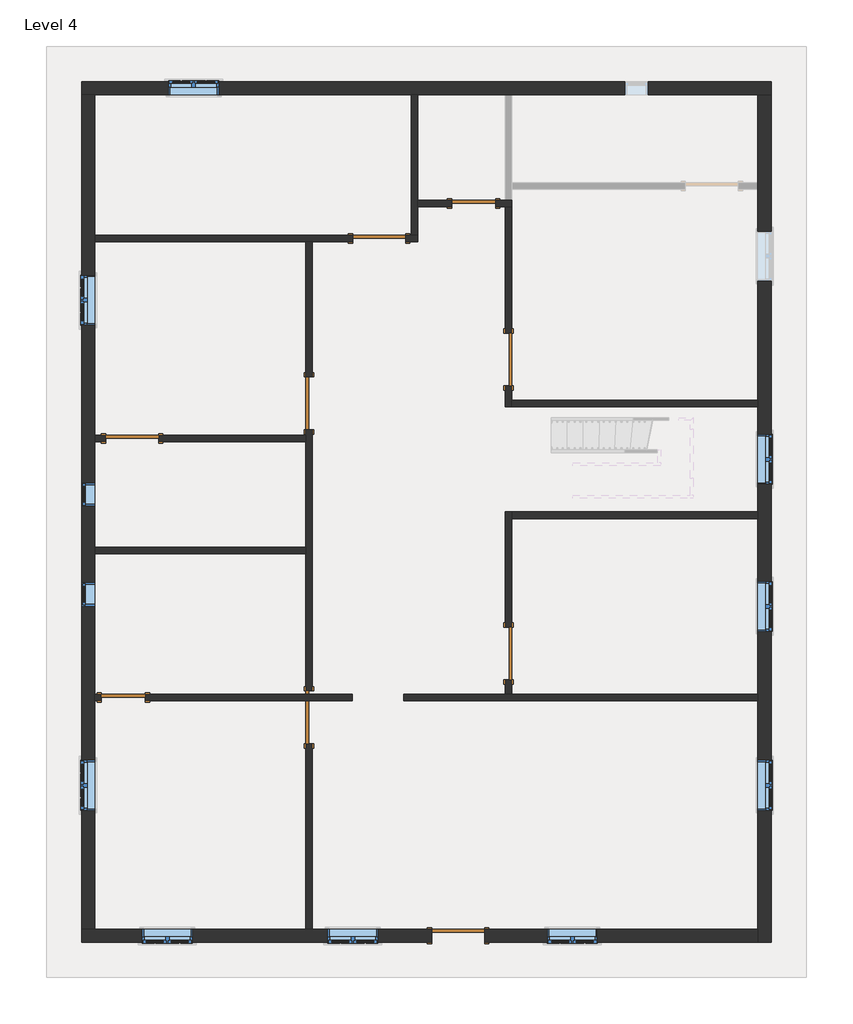
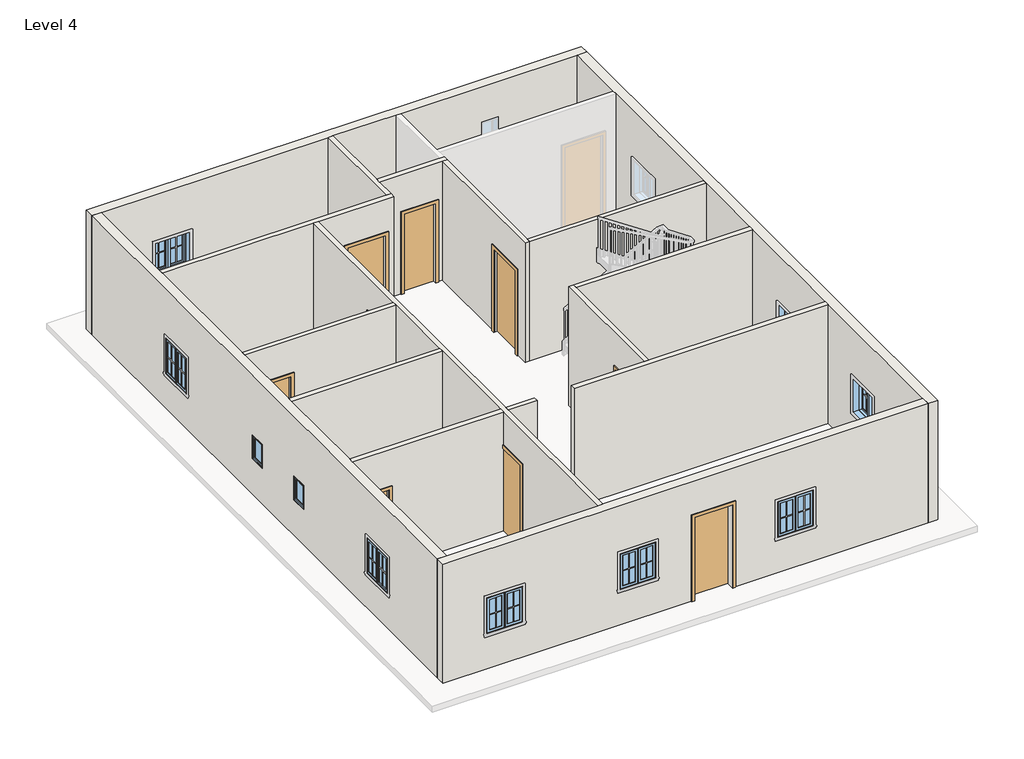
# One storey, part 1 of 3: 16 walls, 11 windows, 9 doors.
"""IFC4 building model written with IfcOpenShell, lengths in millimetres."""

from ifc_helpers import new_model, si_unit, frame, origin, place, context, project, spatial, polyline, outline, extrude, faceted_brep, transform, mapped, element, save
from components import door_d8f5dbb5, door_f2b275c1, door_e5f9f3c4, door_305aa2a5, door_a90ba1ad, window_aa618e30, window_339605e1

model = new_model("IFC4")

# Units and contexts
model_context = context("Model", 3, world=origin())
ifc_project = project(units=[si_unit("LENGTHUNIT", "METRE", prefix="MILLI")], contexts=[model_context])

# Site, building, storey
site = spatial("IfcSite", under=ifc_project)
building = spatial("IfcBuilding", under=site)
storey = spatial("IfcBuildingStorey", under=building, Name="Level 4", Elevation=6400.8)

# Doors
placement = place(None, origin())
door_shape = door_d8f5dbb5(model_context)
element("IfcDoor", 1, ObjectType="Single-Flush : 30\" x 80\"", at=placement, inside=storey, context=model_context, shape_type="MappedRepresentation", body=[
    mapped(door_shape, transform((-509.1743007, 6967.427558, 6400.8), x_axis=(1.0, 0.0, 0.0), y_axis=(0.0, 1.0, 0.0), z_axis=(0.0, 0.0, 1.0))),
])
door_2_shape = door_f2b275c1(model_context)
element("IfcDoor", 2, ObjectType="Single-Flush : 30\" x 80\"", at=placement, inside=storey, context=model_context, shape_type="MappedRepresentation", body=[
    mapped(door_2_shape, transform((-6586.1243007, -1605.072442, 6400.8), x_axis=(-1.0, 0.0, 0.0), y_axis=(0.0, -1.0, 0.0), z_axis=(0.0, 0.0, 1.0))),
])
door_3_shape = door_e5f9f3c4(model_context)
element("IfcDoor", 3, ObjectType="Single-Flush : 36\" x 84\"", at=placement, inside=storey, context=model_context, shape_type="MappedRepresentation", body=[
    mapped(door_3_shape, transform((-2147.4743007, 6357.827558, 6400.8), x_axis=(1.0, 0.0, 0.0), y_axis=(0.0, 1.0, 0.0), z_axis=(0.0, 0.0, 1.0))),
])
element("IfcDoor", 4, ObjectType="Single-Flush : 36\" x 84\"", at=placement, inside=storey, context=model_context, shape_type="MappedRepresentation", body=[
    mapped(door_3_shape, transform((100.4256993, 4262.327558, 6400.8), x_axis=(0.0, -1.0, 0.0), y_axis=(1.0, 0.0, 0.0), z_axis=(0.0, 0.0, 1.0))),
])
element("IfcDoor", 5, ObjectType="Single-Flush : 36\" x 84\"", at=placement, inside=storey, context=model_context, shape_type="MappedRepresentation", body=[
    mapped(door_3_shape, transform((100.4256993, -843.072442, 6400.8), x_axis=(0.0, -1.0, 0.0), y_axis=(1.0, 0.0, 0.0), z_axis=(0.0, 0.0, 1.0))),
])
element("IfcDoor", 6, ObjectType="Single-Flush : 36\" x 84\"", at=placement, inside=storey, context=model_context, shape_type="MappedRepresentation", body=[
    mapped(door_3_shape, transform((-3366.6743007, -1947.972442, 6400.8), x_axis=(0.0, 1.0, 0.0), y_axis=(-1.0, 0.0, 0.0), z_axis=(0.0, 0.0, 1.0))),
])
door_4_shape = door_305aa2a5(model_context)
element("IfcDoor", 7, ObjectType="Single-Flush : 36\" x 84\"", at=placement, inside=storey, context=model_context, shape_type="MappedRepresentation", body=[
    mapped(door_4_shape, transform((-6433.7243007, 2890.727558, 6400.8), x_axis=(-1.0, 0.0, 0.0), y_axis=(0.0, -1.0, 0.0), z_axis=(0.0, 0.0, 1.0))),
])
element("IfcDoor", 8, ObjectType="Single-Flush : 36\" x 84\"", at=placement, inside=storey, context=model_context, shape_type="MappedRepresentation", body=[
    mapped(door_4_shape, transform((-3366.6743007, 3500.327558, 6400.8), x_axis=(0.0, -1.0, 0.0), y_axis=(1.0, 0.0, 0.0), z_axis=(0.0, 0.0, 1.0))),
])
door_5_shape = door_a90ba1ad(model_context)
element("IfcDoor", 9, ObjectType="Single-Flush : 36\" x 84\"", at=placement, inside=storey, context=model_context, shape_type="MappedRepresentation", body=[
    mapped(door_5_shape, transform((-775.8743007, -5738.922442, 6400.8), x_axis=(-1.0, 0.0, 0.0), y_axis=(0.0, -1.0, 0.0), z_axis=(0.0, 0.0, 1.0))),
])

# Walls
element("IfcWall", 10, ObjectType="WALL4.5\"", at=placement, inside=storey, context=model_context, shape_type="Brep", body=[
    faceted_brep([(-1690.2743007, 6300.677558, 8534.4), (-1690.2743007, 6300.677558, 6400.8), (-1480.7243007, 6300.677558, 6400.8), (-1480.7243007, 6300.677558, 9448.8), (-3309.5243007, 6300.677558, 9448.8), (-3423.8243007, 6300.677558, 9448.8), (-7081.4243007, 6300.677558, 9448.8), (-7081.4243007, 6300.677558, 6400.8), (-3423.8243007, 6300.677558, 6400.8), (-3309.5243007, 6300.677558, 6400.8), (-2604.6743007, 6300.677558, 6400.8), (-2604.6743007, 6300.677558, 8534.4), (-1480.7243007, 6414.977558, 6400.8), (-1595.0243007, 6414.977558, 6400.8), (-1690.2743007, 6414.977558, 6400.8), (-1690.2743007, 6414.977558, 8534.4), (-2604.6743007, 6414.977558, 8534.4), (-2604.6743007, 6414.977558, 6400.8), (-7081.4243007, 6414.977558, 6400.8), (-7081.4243007, 6414.977558, 9448.8), (-1595.0243007, 6414.977558, 9448.8), (-1480.7243007, 6414.977558, 9448.8)], [[[0, 1, 2, 3, 4, 5, 6, 7, 8, 9, 10, 11]], [[12, 13, 14, 15, 16, 17, 18, 19, 20, 21]], [[2, 1, 14, 13, 12]], [[10, 9, 8, 7, 18, 17]], [[7, 6, 19, 18]], [[3, 2, 12, 21]], [[15, 14, 1, 0]], [[16, 15, 0, 11]], [[17, 16, 11, 10]], [[6, 5, 4, 3, 21, 20, 19]]]),
])
element("IfcWall", 11, ObjectType="WALL4.5\"", at=placement, inside=storey, context=model_context, shape_type="Brep", body=[
    faceted_brep([(-1480.7243007, 6414.977558, 6400.8), (-1480.7243007, 6910.277558, 6400.8), (-1480.7243007, 7024.577558, 6400.8), (-1480.7243007, 8853.377558, 6400.8), (-1480.7243007, 8853.377558, 9448.8), (-1480.7243007, 7024.577558, 9448.8), (-1480.7243007, 6910.277558, 9448.8), (-1480.7243007, 6414.977558, 9448.8), (-1595.0243007, 6414.977558, 6400.8), (-1595.0243007, 6414.977558, 9448.8), (-1595.0243007, 8853.377558, 9448.8), (-1595.0243007, 8853.377558, 6400.8)], [[[0, 1, 2, 3, 4, 5, 6, 7]], [[8, 9, 10, 11]], [[3, 2, 1, 0, 8, 11]], [[0, 7, 9, 8]], [[4, 3, 11, 10]], [[7, 6, 5, 4, 10, 9]]]),
])
element("IfcWall", 12, ObjectType="WALL4.5\"", at=placement, inside=storey, context=model_context, shape_type="Brep", body=[
    faceted_brep([(-128.1743007, 6910.277558, 8432.8), (-128.1743007, 6910.277558, 6400.8), (43.2756993, 6910.277558, 6400.8), (157.5756993, 6910.277558, 6400.8), (157.5756993, 6910.277558, 9448.8), (43.2756993, 6910.277558, 9448.8), (-1480.7243007, 6910.277558, 9448.8), (-1480.7243007, 6910.277558, 6400.8), (-890.1743007, 6910.277558, 6400.8), (-890.1743007, 6910.277558, 8432.8), (157.5756993, 7024.577558, 6400.8), (43.2756993, 7024.577558, 6400.8), (-128.1743007, 7024.577558, 6400.8), (-128.1743007, 7024.577558, 8432.8), (-890.1743007, 7024.577558, 8432.8), (-890.1743007, 7024.577558, 6400.8), (-1480.7243007, 7024.577558, 6400.8), (-1480.7243007, 7024.577558, 9448.8), (43.2756993, 7024.577558, 9448.8), (157.5756993, 7024.577558, 9448.8)], [[[0, 1, 2, 3, 4, 5, 6, 7, 8, 9]], [[10, 11, 12, 13, 14, 15, 16, 17, 18, 19]], [[8, 7, 16, 15]], [[3, 2, 1, 12, 11, 10]], [[7, 6, 17, 16]], [[4, 3, 10, 19]], [[13, 12, 1, 0]], [[14, 13, 0, 9]], [[15, 14, 9, 8]], [[6, 5, 4, 19, 18, 17]]]),
])
element("IfcWall", 13, ObjectType="WALL4.5\"", at=placement, inside=storey, context=model_context, shape_type="Brep", body=[
    faceted_brep([(-3423.8243007, 3043.127558, 6400.8), (-3423.8243007, 2947.877558, 6400.8), (-3423.8243007, 2833.577558, 6400.8), (-3423.8243007, 1004.777558, 6400.8), (-3423.8243007, 890.477558, 6400.8), (-3423.8243007, -1490.772442, 6400.8), (-3423.8243007, -1490.772442, 8534.4), (-3423.8243007, -1547.922442, 8534.4), (-3423.8243007, -1662.222442, 8534.4), (-3423.8243007, -2405.172442, 8534.4), (-3423.8243007, -2405.172442, 6400.8), (-3423.8243007, -5624.622442, 6400.8), (-3423.8243007, -5624.622442, 9448.8), (-3423.8243007, -1662.222442, 9448.8), (-3423.8243007, -1547.922442, 9448.8), (-3423.8243007, 890.477558, 9448.8), (-3423.8243007, 1004.777558, 9448.8), (-3423.8243007, 2833.577558, 9448.8), (-3423.8243007, 2947.877558, 9448.8), (-3423.8243007, 6300.677558, 9448.8), (-3423.8243007, 6300.677558, 6400.8), (-3423.8243007, 3957.527558, 6400.8), (-3423.8243007, 3957.527558, 8534.4), (-3423.8243007, 3043.127558, 8534.4), (-3309.5243007, -1490.772442, 8534.4), (-3309.5243007, -1490.772442, 6400.8), (-3309.5243007, 3043.127558, 6400.8), (-3309.5243007, 3043.127558, 8534.4), (-3309.5243007, 3957.527558, 8534.4), (-3309.5243007, 3957.527558, 6400.8), (-3309.5243007, 6300.677558, 6400.8), (-3309.5243007, 6300.677558, 9448.8), (-3309.5243007, -1547.922442, 9448.8), (-3309.5243007, -1662.222442, 9448.8), (-3309.5243007, -5624.622442, 9448.8), (-3309.5243007, -5624.622442, 6400.8), (-3309.5243007, -2405.172442, 6400.8), (-3309.5243007, -2405.172442, 8534.4), (-3309.5243007, -1662.222442, 8534.4), (-3309.5243007, -1547.922442, 8534.4)], [[[0, 1, 2, 3, 4, 5, 6, 7, 8, 9, 10, 11, 12, 13, 14, 15, 16, 17, 18, 19, 20, 21, 22, 23]], [[24, 25, 26, 27, 28, 29, 30, 31, 32, 33, 34, 35, 36, 37, 38, 39]], [[21, 20, 30, 29]], [[36, 35, 11, 10]], [[26, 25, 5, 4, 3, 2, 1, 0]], [[12, 11, 35, 34]], [[20, 19, 31, 30]], [[27, 26, 0, 23]], [[28, 27, 23, 22]], [[29, 28, 22, 21]], [[6, 5, 25, 24]], [[9, 8, 7, 6, 24, 39, 38, 37]], [[10, 9, 37, 36]], [[19, 18, 17, 16, 15, 14, 13, 12, 34, 33, 32, 31]]]),
])
element("IfcWall", 14, ObjectType="WALL4.5\"", at=placement, inside=storey, context=model_context, shape_type="Brep", body=[
    faceted_brep([(157.5756993, -1547.922442, 6400.8), (157.5756993, -1300.272442, 6400.8), (157.5756993, -1300.272442, 8534.4), (157.5756993, -385.872442, 8534.4), (157.5756993, -385.872442, 6400.8), (157.5756993, 1500.077558, 6400.8), (157.5756993, 1614.377558, 6400.8), (157.5756993, 1614.377558, 9448.8), (157.5756993, 1500.077558, 9448.8), (157.5756993, -1547.922442, 9448.8), (43.2756993, -1300.272442, 8534.4), (43.2756993, -1300.272442, 6400.8), (43.2756993, -1547.922442, 6400.8), (43.2756993, -1547.922442, 9448.8), (43.2756993, 1614.377558, 9448.8), (43.2756993, 1614.377558, 6400.8), (43.2756993, -385.872442, 6400.8), (43.2756993, -385.872442, 8534.4)], [[[0, 1, 2, 3, 4, 5, 6, 7, 8, 9]], [[10, 11, 12, 13, 14, 15, 16, 17]], [[16, 15, 6, 5, 4]], [[12, 11, 1, 0]], [[7, 6, 15, 14]], [[0, 9, 13, 12]], [[2, 1, 11, 10]], [[3, 2, 10, 17]], [[4, 3, 17, 16]], [[9, 8, 7, 14, 13]]]),
])
element("IfcWall", 15, ObjectType="WALL4.5\"", at=placement, inside=storey, context=model_context, shape_type="SweptSolid", body=[
    extrude(outline(polyline([(4424.7756993, 1500.077558), (157.5756993, 1500.077558), (157.5756993, 1614.377558), (4424.7756993, 1614.377558), (4424.7756993, 1500.077558)])), frame((0.0, 0.0, 6400.8), z_axis=(0.0, 0.0, 1.0), x_axis=(1.0, 0.0, 0.0)), (0.0, 0.0, 1.0), 3048.0),
])
element("IfcWall", 16, ObjectType="WALL4.5\"", at=placement, inside=storey, context=model_context, shape_type="SweptSolid", body=[
    extrude(outline(polyline([(-3423.8243007, 890.477558), (-7081.4243007, 890.477558), (-7081.4243007, 1004.777558), (-3423.8243007, 1004.777558), (-3423.8243007, 890.477558)])), frame((0.0, 0.0, 6400.8), z_axis=(0.0, 0.0, 1.0), x_axis=(1.0, 0.0, 0.0)), (0.0, 0.0, 1.0), 3048.0),
])
element("IfcWall", 17, ObjectType="WALL4.5\"", at=placement, inside=storey, context=model_context, shape_type="SweptSolid", body=[
    extrude(outline(polyline([(6400.8, -7081.4243007), (6400.8, -6890.9243007), (8534.4, -6890.9243007), (8534.4, -5976.5243007), (6400.8, -5976.5243007), (6400.8, -3423.8243007), (9448.8, -3423.8243007), (9448.8, -7081.4243007), (6400.8, -7081.4243007)])), frame((0.0, 2833.577558, 0.0), z_axis=(0.0, 1.0, 0.0), x_axis=(0.0, 0.0, 1.0)), (0.0, 0.0, 1.0), 114.3),
])
element("IfcWall", 18, ObjectType="WALL4.5\"", at=placement, inside=storey, context=model_context, shape_type="Brep", body=[
    faceted_brep([(43.2756993, 3805.127558, 8534.4), (43.2756993, 3805.127558, 6400.8), (43.2756993, 3443.177558, 6400.8), (43.2756993, 3443.177558, 9448.8), (43.2756993, 6910.277558, 9448.8), (43.2756993, 6910.277558, 6400.8), (43.2756993, 4719.527558, 6400.8), (43.2756993, 4719.527558, 8534.4), (157.5756993, 3443.177558, 6400.8), (157.5756993, 3557.477558, 6400.8), (157.5756993, 3805.127558, 6400.8), (157.5756993, 3805.127558, 8534.4), (157.5756993, 4719.527558, 8534.4), (157.5756993, 4719.527558, 6400.8), (157.5756993, 6910.277558, 6400.8), (157.5756993, 6910.277558, 9448.8), (157.5756993, 3557.477558, 9448.8), (157.5756993, 3443.177558, 9448.8)], [[[0, 1, 2, 3, 4, 5, 6, 7]], [[8, 9, 10, 11, 12, 13, 14, 15, 16, 17]], [[6, 5, 14, 13]], [[2, 1, 10, 9, 8]], [[5, 4, 15, 14]], [[3, 2, 8, 17]], [[11, 10, 1, 0]], [[12, 11, 0, 7]], [[13, 12, 7, 6]], [[4, 3, 17, 16, 15]]]),
])
element("IfcWall", 19, ObjectType="WALL4.5\"", at=placement, inside=storey, context=model_context, shape_type="SweptSolid", body=[
    extrude(outline(polyline([(4424.7756993, 3443.177558), (157.5756993, 3443.177558), (157.5756993, 3557.477558), (4424.7756993, 3557.477558), (4424.7756993, 3443.177558)])), frame((0.0, 0.0, 6400.8), z_axis=(0.0, 0.0, 1.0), x_axis=(1.0, 0.0, 0.0)), (0.0, 0.0, 1.0), 3048.0),
])
element("IfcWall", 20, ObjectType="WALL4.5\"", at=placement, inside=storey, context=model_context, shape_type="SweptSolid", body=[
    extrude(outline(polyline([(6400.8, -2614.8628774), (9448.8, -2614.8628774), (9448.8, -3309.5243007), (8534.4, -3309.5243007), (8534.4, -3423.8243007), (9448.8, -3423.8243007), (9448.8, -7081.4243007), (6400.8, -7081.4243007), (6400.8, -6967.1243007), (8432.8, -6967.1243007), (8432.8, -6205.1243007), (6400.8, -6205.1243007), (6400.8, -2614.8628774)])), frame((0.0, -1662.222442, 0.0), z_axis=(0.0, 1.0, 0.0), x_axis=(0.0, 0.0, 1.0)), (0.0, 0.0, 1.0), 114.3),
])
element("IfcWall", 21, ObjectType="WALL4.5\"", at=placement, inside=storey, context=model_context, shape_type="Brep", body=[
    faceted_brep([(-1720.6441625, -1662.222442, 6400.8), (4424.7756993, -1662.222442, 6400.8), (4424.7756993, -1662.222442, 9448.8), (-1720.6441625, -1662.222442, 9448.8), (-1720.6441625, -1547.922442, 6400.8), (-1720.6441625, -1547.922442, 9448.8), (43.2756993, -1547.922442, 9448.8), (157.5756993, -1547.922442, 9448.8), (4424.7756993, -1547.922442, 9448.8), (4424.7756993, -1547.922442, 6400.8), (157.5756993, -1547.922442, 6400.8), (43.2756993, -1547.922442, 6400.8)], [[[0, 1, 2, 3]], [[4, 5, 6, 7, 8, 9, 10, 11]], [[1, 0, 4, 11, 10, 9]], [[0, 3, 5, 4]], [[2, 1, 9, 8]], [[3, 2, 8, 7, 6, 5]]]),
])
element("IfcWall", 22, ObjectType="WALL9\"", at=placement, inside=storey, context=model_context, shape_type="Brep", body=[
    faceted_brep([(-7310.0243007, 8853.377558, 6400.8), (-7081.4243007, 8853.377558, 6400.8), (-1595.0243007, 8853.377558, 6400.8), (-1480.7243007, 8853.377558, 6400.8), (43.2756993, 8853.377558, 6400.8), (157.5756993, 8853.377558, 6400.8), (4424.7756993, 8853.377558, 6400.8), (4653.3756993, 8853.377558, 6400.8), (4653.3756993, 8853.377558, 9448.8), (4424.7756993, 8853.377558, 9448.8), (157.5756993, 8853.377558, 9448.8), (43.2756993, 8853.377558, 9448.8), (-1480.7243007, 8853.377558, 9448.8), (-1595.0243007, 8853.377558, 9448.8), (-7081.4243007, 8853.377558, 9448.8), (-7310.0243007, 8853.377558, 9448.8), (-4935.1243007, 8853.377558, 8229.6), (-4935.1243007, 8853.377558, 7315.2), (-5798.7243007, 8853.377558, 7315.2), (-5798.7243007, 8853.377558, 8229.6), (2522.9506993, 8853.377558, 8534.4), (2522.9506993, 8853.377558, 6705.6), (2116.5506993, 8853.377558, 6705.6), (2116.5506993, 8853.377558, 8534.4), (-7310.0243007, 9081.977558, 6400.8), (-7310.0243007, 9081.977558, 9448.8), (4653.3756993, 9081.977558, 9448.8), (4653.3756993, 9081.977558, 6400.8), (-4935.1243007, 9081.977558, 8229.6), (-5798.7243007, 9081.977558, 8229.6), (-5798.7243007, 9081.977558, 7315.2), (-4935.1243007, 9081.977558, 7315.2), (2522.9506993, 9081.977558, 8534.4), (2116.5506993, 9081.977558, 8534.4), (2116.5506993, 9081.977558, 6705.6), (2522.9506993, 9081.977558, 6705.6)], [[[0, 1, 2, 3, 4, 5, 6, 7, 8, 9, 10, 11, 12, 13, 14, 15], [16, 17, 18, 19], [20, 21, 22, 23]], [[24, 25, 26, 27], [28, 29, 30, 31], [32, 33, 34, 35]], [[7, 6, 5, 4, 3, 2, 1, 0, 24, 27]], [[8, 7, 27, 26]], [[0, 15, 25, 24]], [[17, 16, 28, 31]], [[18, 17, 31, 30]], [[19, 18, 30, 29]], [[16, 19, 29, 28]], [[21, 20, 32, 35]], [[22, 21, 35, 34]], [[23, 22, 34, 33]], [[20, 23, 33, 32]], [[15, 14, 13, 12, 11, 10, 9, 8, 26, 25]]]),
])
element("IfcWall", 23, ObjectType="WALL9\"", at=placement, inside=storey, context=model_context, shape_type="Brep", body=[
    faceted_brep([(4424.7756993, 8853.377558, 6400.8), (4424.7756993, 7329.377558, 6400.8), (4424.7756993, 7215.077558, 6400.8), (4424.7756993, 3557.477558, 6400.8), (4424.7756993, 3443.177558, 6400.8), (4424.7756993, 1614.377558, 6400.8), (4424.7756993, 1500.077558, 6400.8), (4424.7756993, -1547.922442, 6400.8), (4424.7756993, -1662.222442, 6400.8), (4424.7756993, -5624.622442, 6400.8), (4424.7756993, -5853.222442, 6400.8), (4424.7756993, -5853.222442, 9448.8), (4424.7756993, -5624.622442, 9448.8), (4424.7756993, -1662.222442, 9448.8), (4424.7756993, -1547.922442, 9448.8), (4424.7756993, 1500.077558, 9448.8), (4424.7756993, 1614.377558, 9448.8), (4424.7756993, 3443.177558, 9448.8), (4424.7756993, 3557.477558, 9448.8), (4424.7756993, 7215.077558, 9448.8), (4424.7756993, 7329.377558, 9448.8), (4424.7756993, 8853.377558, 9448.8), (4424.7756993, 5621.227558, 8229.6), (4424.7756993, 5621.227558, 7315.2), (4424.7756993, 6484.827558, 7315.2), (4424.7756993, 6484.827558, 8229.6), (4424.7756993, 2096.977558, 8229.6), (4424.7756993, 2096.977558, 7315.2), (4424.7756993, 2960.577558, 7315.2), (4424.7756993, 2960.577558, 8229.6), (4424.7756993, -455.722442, 8229.6), (4424.7756993, -455.722442, 7315.2), (4424.7756993, 407.877558, 7315.2), (4424.7756993, 407.877558, 8229.6), (4424.7756993, -3560.872442, 8229.6), (4424.7756993, -3560.872442, 7315.2), (4424.7756993, -2697.272442, 7315.2), (4424.7756993, -2697.272442, 8229.6), (4653.3756993, 8853.377558, 6400.8), (4653.3756993, 8853.377558, 9448.8), (4653.3756993, -5853.222442, 9448.8), (4653.3756993, -5853.222442, 6400.8), (4653.3756993, 5621.227558, 8229.6), (4653.3756993, 6484.827558, 8229.6), (4653.3756993, 6484.827558, 7315.2), (4653.3756993, 5621.227558, 7315.2), (4653.3756993, 2096.977558, 8229.6), (4653.3756993, 2960.577558, 8229.6), (4653.3756993, 2960.577558, 7315.2), (4653.3756993, 2096.977558, 7315.2), (4653.3756993, -455.722442, 8229.6), (4653.3756993, 407.877558, 8229.6), (4653.3756993, 407.877558, 7315.2), (4653.3756993, -455.722442, 7315.2), (4653.3756993, -3560.872442, 8229.6), (4653.3756993, -2697.272442, 8229.6), (4653.3756993, -2697.272442, 7315.2), (4653.3756993, -3560.872442, 7315.2)], [[[0, 1, 2, 3, 4, 5, 6, 7, 8, 9, 10, 11, 12, 13, 14, 15, 16, 17, 18, 19, 20, 21], [22, 23, 24, 25], [26, 27, 28, 29], [30, 31, 32, 33], [34, 35, 36, 37]], [[38, 39, 40, 41], [42, 43, 44, 45], [46, 47, 48, 49], [50, 51, 52, 53], [54, 55, 56, 57]], [[10, 9, 8, 7, 6, 5, 4, 3, 2, 1, 0, 38, 41]], [[0, 21, 39, 38]], [[11, 10, 41, 40]], [[23, 22, 42, 45]], [[24, 23, 45, 44]], [[25, 24, 44, 43]], [[22, 25, 43, 42]], [[27, 26, 46, 49]], [[28, 27, 49, 48]], [[29, 28, 48, 47]], [[26, 29, 47, 46]], [[31, 30, 50, 53]], [[32, 31, 53, 52]], [[33, 32, 52, 51]], [[30, 33, 51, 50]], [[35, 34, 54, 57]], [[36, 35, 57, 56]], [[37, 36, 56, 55]], [[34, 37, 55, 54]], [[21, 20, 19, 18, 17, 16, 15, 14, 13, 12, 11, 40, 39]]]),
])
element("IfcWall", 24, ObjectType="WALL9\"", at=placement, inside=storey, context=model_context, shape_type="Brep", body=[
    faceted_brep([(-1233.0743007, -5624.622442, 8534.4), (-1233.0743007, -5624.622442, 6400.8), (-3309.5243007, -5624.622442, 6400.8), (-3423.8243007, -5624.622442, 6400.8), (-7081.4243007, -5624.622442, 6400.8), (-7310.0243007, -5624.622442, 6400.8), (-7310.0243007, -5624.622442, 9448.8), (-7081.4243007, -5624.622442, 9448.8), (-3423.8243007, -5624.622442, 9448.8), (-3309.5243007, -5624.622442, 9448.8), (4424.7756993, -5624.622442, 9448.8), (4424.7756993, -5624.622442, 6400.8), (-318.6743007, -5624.622442, 6400.8), (-318.6743007, -5624.622442, 8534.4), (773.5256993, -5624.622442, 8229.6), (773.5256993, -5624.622442, 7315.2), (1637.1256993, -5624.622442, 7315.2), (1637.1256993, -5624.622442, 8229.6), (-3036.4743007, -5624.622442, 8229.6), (-3036.4743007, -5624.622442, 7315.2), (-2172.8743007, -5624.622442, 7315.2), (-2172.8743007, -5624.622442, 8229.6), (-6255.9243007, -5624.622442, 8229.6), (-6255.9243007, -5624.622442, 7315.2), (-5392.3243007, -5624.622442, 7315.2), (-5392.3243007, -5624.622442, 8229.6), (-7310.0243007, -5853.222442, 6400.8), (-1233.0743007, -5853.222442, 6400.8), (-1233.0743007, -5853.222442, 8534.4), (-318.6743007, -5853.222442, 8534.4), (-318.6743007, -5853.222442, 6400.8), (4424.7756993, -5853.222442, 6400.8), (4424.7756993, -5853.222442, 9448.8), (-7310.0243007, -5853.222442, 9448.8), (773.5256993, -5853.222442, 8229.6), (1637.1256993, -5853.222442, 8229.6), (1637.1256993, -5853.222442, 7315.2), (773.5256993, -5853.222442, 7315.2), (-3036.4743007, -5853.222442, 8229.6), (-2172.8743007, -5853.222442, 8229.6), (-2172.8743007, -5853.222442, 7315.2), (-3036.4743007, -5853.222442, 7315.2), (-6255.9243007, -5853.222442, 8229.6), (-5392.3243007, -5853.222442, 8229.6), (-5392.3243007, -5853.222442, 7315.2), (-6255.9243007, -5853.222442, 7315.2)], [[[0, 1, 2, 3, 4, 5, 6, 7, 8, 9, 10, 11, 12, 13], [14, 15, 16, 17], [18, 19, 20, 21], [22, 23, 24, 25]], [[26, 27, 28, 29, 30, 31, 32, 33], [34, 35, 36, 37], [38, 39, 40, 41], [42, 43, 44, 45]], [[12, 11, 31, 30]], [[5, 4, 3, 2, 1, 27, 26]], [[11, 10, 32, 31]], [[6, 5, 26, 33]], [[28, 27, 1, 0]], [[29, 28, 0, 13]], [[30, 29, 13, 12]], [[15, 14, 34, 37]], [[16, 15, 37, 36]], [[17, 16, 36, 35]], [[14, 17, 35, 34]], [[19, 18, 38, 41]], [[20, 19, 41, 40]], [[21, 20, 40, 39]], [[18, 21, 39, 38]], [[23, 22, 42, 45]], [[24, 23, 45, 44]], [[25, 24, 44, 43]], [[22, 25, 43, 42]], [[10, 9, 8, 7, 6, 33, 32]]]),
])
element("IfcWall", 25, ObjectType="WALL9\"", at=placement, inside=storey, context=model_context, shape_type="Brep", body=[
    faceted_brep([(-7081.4243007, -5624.622442, 6400.8), (-7081.4243007, -1662.222442, 6400.8), (-7081.4243007, -1547.922442, 6400.8), (-7081.4243007, 890.477558, 6400.8), (-7081.4243007, 1004.777558, 6400.8), (-7081.4243007, 2833.577558, 6400.8), (-7081.4243007, 2947.877558, 6400.8), (-7081.4243007, 6300.677558, 6400.8), (-7081.4243007, 6414.977558, 6400.8), (-7081.4243007, 8853.377558, 6400.8), (-7081.4243007, 8853.377558, 9448.8), (-7081.4243007, 6414.977558, 9448.8), (-7081.4243007, 6300.677558, 9448.8), (-7081.4243007, 2947.877558, 9448.8), (-7081.4243007, 2833.577558, 9448.8), (-7081.4243007, 1004.777558, 9448.8), (-7081.4243007, 890.477558, 9448.8), (-7081.4243007, -1547.922442, 9448.8), (-7081.4243007, -1662.222442, 9448.8), (-7081.4243007, -5624.622442, 9448.8), (-7081.4243007, 388.827558, 7924.8), (-7081.4243007, 388.827558, 7315.2), (-7081.4243007, -17.572442, 7315.2), (-7081.4243007, -17.572442, 7924.8), (-7081.4243007, 2122.377558, 7924.8), (-7081.4243007, 2122.377558, 7315.2), (-7081.4243007, 1715.977558, 7315.2), (-7081.4243007, 1715.977558, 7924.8), (-7081.4243007, 5722.827558, 8229.6), (-7081.4243007, 5722.827558, 7315.2), (-7081.4243007, 4859.227558, 7315.2), (-7081.4243007, 4859.227558, 8229.6), (-7081.4243007, -2697.272442, 8229.6), (-7081.4243007, -2697.272442, 7315.2), (-7081.4243007, -3560.872442, 7315.2), (-7081.4243007, -3560.872442, 8229.6), (-7310.0243007, -5624.622442, 6400.8), (-7310.0243007, -5624.622442, 9448.8), (-7310.0243007, 8853.377558, 9448.8), (-7310.0243007, 8853.377558, 6400.8), (-7310.0243007, 388.827558, 7924.8), (-7310.0243007, -17.572442, 7924.8), (-7310.0243007, -17.572442, 7315.2), (-7310.0243007, 388.827558, 7315.2), (-7310.0243007, 2122.377558, 7924.8), (-7310.0243007, 1715.977558, 7924.8), (-7310.0243007, 1715.977558, 7315.2), (-7310.0243007, 2122.377558, 7315.2), (-7310.0243007, 5722.827558, 8229.6), (-7310.0243007, 4859.227558, 8229.6), (-7310.0243007, 4859.227558, 7315.2), (-7310.0243007, 5722.827558, 7315.2), (-7310.0243007, -2697.272442, 8229.6), (-7310.0243007, -3560.872442, 8229.6), (-7310.0243007, -3560.872442, 7315.2), (-7310.0243007, -2697.272442, 7315.2)], [[[0, 1, 2, 3, 4, 5, 6, 7, 8, 9, 10, 11, 12, 13, 14, 15, 16, 17, 18, 19], [20, 21, 22, 23], [24, 25, 26, 27], [28, 29, 30, 31], [32, 33, 34, 35]], [[36, 37, 38, 39], [40, 41, 42, 43], [44, 45, 46, 47], [48, 49, 50, 51], [52, 53, 54, 55]], [[9, 8, 7, 6, 5, 4, 3, 2, 1, 0, 36, 39]], [[10, 9, 39, 38]], [[0, 19, 37, 36]], [[21, 20, 40, 43]], [[22, 21, 43, 42]], [[23, 22, 42, 41]], [[20, 23, 41, 40]], [[25, 24, 44, 47]], [[26, 25, 47, 46]], [[27, 26, 46, 45]], [[24, 27, 45, 44]], [[29, 28, 48, 51]], [[30, 29, 51, 50]], [[31, 30, 50, 49]], [[28, 31, 49, 48]], [[33, 32, 52, 55]], [[34, 33, 55, 54]], [[35, 34, 54, 53]], [[32, 35, 53, 52]], [[19, 18, 17, 16, 15, 14, 13, 12, 11, 10, 38, 37]]]),
])

# Windows
window_shape = window_aa618e30(model_context)
element("IfcWindow", 26, ObjectType="Fixed : 16\" x 24\"", at=placement, inside=storey, context=model_context, shape_type="MappedRepresentation", body=[
    mapped(window_shape, transform((-7195.7243007, 223.727558, 6400.8), x_axis=(0.0, 1.0, 0.0), y_axis=(-1.0, 0.0, 0.0), z_axis=(0.0, 0.0, 1.0))),
])
element("IfcWindow", 27, ObjectType="Fixed : 16\" x 24\"", at=placement, inside=storey, context=model_context, shape_type="MappedRepresentation", body=[
    mapped(window_shape, transform((-7195.7243007, 1957.277558, 6400.8), x_axis=(0.0, 1.0, 0.0), y_axis=(-1.0, 0.0, 0.0), z_axis=(0.0, 0.0, 1.0))),
])
window_2_shape = window_339605e1(model_context)
element("IfcWindow", 28, ObjectType="Window-Casement-Double : 34\" x 36\"", at=placement, inside=storey, context=model_context, shape_type="MappedRepresentation", body=[
    mapped(window_2_shape, transform((-5366.9243007, 8967.677558, 6400.8), x_axis=(1.0, 0.0, 0.0), y_axis=(0.0, 1.0, 0.0), z_axis=(0.0, 0.0, 1.0))),
])
element("IfcWindow", 29, ObjectType="Window-Casement-Double : 34\" x 36\"", at=placement, inside=storey, context=model_context, shape_type="MappedRepresentation", body=[
    mapped(window_2_shape, transform((-7195.7243007, 5291.027558, 6400.8), x_axis=(0.0, 1.0, 0.0), y_axis=(-1.0, 0.0, 0.0), z_axis=(0.0, 0.0, 1.0))),
])
element("IfcWindow", 30, ObjectType="Window-Casement-Double : 34\" x 36\"", at=placement, inside=storey, context=model_context, shape_type="MappedRepresentation", body=[
    mapped(window_2_shape, transform((4539.0756993, 2528.777558, 6400.8), x_axis=(0.0, -1.0, 0.0), y_axis=(1.0, 0.0, 0.0), z_axis=(0.0, 0.0, 1.0))),
])
element("IfcWindow", 31, ObjectType="Window-Casement-Double : 34\" x 36\"", at=placement, inside=storey, context=model_context, shape_type="MappedRepresentation", body=[
    mapped(window_2_shape, transform((4539.0756993, -23.922442, 6400.8), x_axis=(0.0, -1.0, 0.0), y_axis=(1.0, 0.0, 0.0), z_axis=(0.0, 0.0, 1.0))),
])
element("IfcWindow", 32, ObjectType="Window-Casement-Double : 34\" x 36\"", at=placement, inside=storey, context=model_context, shape_type="MappedRepresentation", body=[
    mapped(window_2_shape, transform((4539.0756993, -3129.072442, 6400.8), x_axis=(0.0, -1.0, 0.0), y_axis=(1.0, 0.0, 0.0), z_axis=(0.0, 0.0, 1.0))),
])
element("IfcWindow", 33, ObjectType="Window-Casement-Double : 34\" x 36\"", at=placement, inside=storey, context=model_context, shape_type="MappedRepresentation", body=[
    mapped(window_2_shape, transform((1205.3256993, -5738.922442, 6400.8), x_axis=(-1.0, 0.0, 0.0), y_axis=(0.0, -1.0, 0.0), z_axis=(0.0, 0.0, 1.0))),
])
element("IfcWindow", 34, ObjectType="Window-Casement-Double : 34\" x 36\"", at=placement, inside=storey, context=model_context, shape_type="MappedRepresentation", body=[
    mapped(window_2_shape, transform((-2604.6743007, -5738.922442, 6400.8), x_axis=(-1.0, 0.0, 0.0), y_axis=(0.0, -1.0, 0.0), z_axis=(0.0, 0.0, 1.0))),
])
element("IfcWindow", 35, ObjectType="Window-Casement-Double : 34\" x 36\"", at=placement, inside=storey, context=model_context, shape_type="MappedRepresentation", body=[
    mapped(window_2_shape, transform((-5824.1243007, -5738.922442, 6400.8), x_axis=(-1.0, 0.0, 0.0), y_axis=(0.0, -1.0, 0.0), z_axis=(0.0, 0.0, 1.0))),
])
element("IfcWindow", 36, ObjectType="Window-Casement-Double : 34\" x 36\"", at=placement, inside=storey, context=model_context, shape_type="MappedRepresentation", body=[
    mapped(window_2_shape, transform((-7195.7243007, -3129.072442, 6400.8), x_axis=(0.0, 1.0, 0.0), y_axis=(-1.0, 0.0, 0.0), z_axis=(0.0, 0.0, 1.0))),
])

save(model, "model.ifc")

# Revit data of these elements
# Type "Single-Flush : 30\" x 80\""
#   Type Mark = "5"
#   Construction Type Id = "MDOOR"
#   Assembly Code = "C1020"
#   Analytic Construction = "Metal"
#   Thickness = 0' - 2"
#   Heat Transfer Coefficient (U) = 0.651978 BTU/(h·ft²·°F)
#   Height = 6' - 8"
#   Trim Projection Ext = 0' - 1"
#   Trim Projection Int = 0' - 1"
#   Trim Width = 0' - 3"
#   Width = 2' - 6"
#   Define Thermal Properties by = 1
#   Define Thermal Properties by = 1
#   Door Material = Door - Panel
#   Frame Material = Door - Frame
#   Visual Light Transmittance = 0
#   Solar Heat Gain Coefficient = 0
#   Function = (empty or 0)
#   Wall Closure = (empty or 0)
# Type "Single-Flush : 36\" x 84\""
#   Type Mark = "1"
#   Construction Type Id = "MDOOR"
#   Assembly Code = "C1020"
#   Analytic Construction = "Metal"
#   Thickness = 0' - 2"
#   Heat Transfer Coefficient (U) = 0.651978 BTU/(h·ft²·°F)
#   Height = 7' - 0"
#   Trim Projection Ext = 0' - 1"
#   Trim Projection Int = 0' - 1"
#   Trim Width = 0' - 3"
#   Width = 3' - 0"
#   Define Thermal Properties by = 1
#   Define Thermal Properties by = 1
#   Door Material = Door - Panel
#   Frame Material = Door - Frame
#   Visual Light Transmittance = 0
#   Solar Heat Gain Coefficient = 0
#   Function = (empty or 0)
#   Wall Closure = (empty or 0)
# Type "WALL4.5\""
#   Assembly Code = "B2010"
#   Layers, outside or top first: 0' - 4 1/2" no material (function 1)
# Type "WALL9\""
#   Assembly Code = "B2010"
#   Layers, outside or top first: 0' - 9" no material (function 1)
# Type "Fixed : 16\" x 24\""
#   Type Mark = "4"
#   Construction Type Id = "GSP4R"
#   Assembly Code = "B2020100"
#   Analytic Construction = "1/8 in Pilkington single glazing"
#   Visual Light Transmittance = 0.9
#   Solar Heat Gain Coefficient = 0.78
#   Heat Transfer Coefficient (U) = 0.6496 BTU/(h·ft²·°F)
#   Height = 2' - 0"
#   Default Sill Height = 3' - 0"
#   Width = 1' - 4"
#   Window Inset = 0' - 0 3/4"
#   Define Thermal Properties by = 1
#   Define Thermal Properties by = 1
#   Glass Pane Material = Glass
#   Sash Material = Sash
#   Wall Closure = (empty or 0)
# Type "Window-Casement-Double : 34\" x 36\""
#   Type Mark = "14"
#   Fire Rating = "0.5h"
#   Assembly Code = "B2020100"
#   Analytic Construction = "Double glazing - domestic"
#   Frame Extension [instance default] = 0' - 0 1/4"
#   Window Inset [instance default] = 0' - 0"
#   Wall Thickness [instance default] = 0' - 6"
#   Interior Wall Closure [instance default] = 0' - 2 1/4"
#   Half Width = 1' - 5"
#   Visual Light Transmittance = 0.81
#   Thermal Resistance (R) = 1.8146 (h·ft²·°F)/BTU
#   Solar Heat Gain Coefficient = 0.76
#   Rough Width = 2' - 10 1/2"
#   Rough Height = 3' - 0 1/2"
#   Height = 3' - 0"
#   Heat Transfer Coefficient (U) = 0.5511 BTU/(h·ft²·°F)
#   Exterior Wall Closure [instance default] = 0' - 1 1/4"
#   Extension Jamb [instance default] = 0' - 2 1/4"
#   Default Sill Height = 3' - 0"
#   Width = 2' - 10"
#   Define Thermal Properties by = 0
#   Muntin Visibility = yes
#   Interior Trim Visibility [instance default] = yes
#   Exterior Trim Visibility [instance default] = yes
#   Extension Jamb Visibility [instance default] = yes
#   Interior Trim Material = Wood - Stained
#   Muntin Pattern = Muntin Pattern_2x2 : Muntin Pattern_2x2
#   Interior Trim = Trim-Window-Interior-Flat : Picture Frame
#   Interior Frame Material = Wood - Stained
#   Glass Panel Material = Glass
#   Exterior Trim Material = Clad - White
#   Exterior Trim = Trim-Window-Exterior-Flat : with Sill
#   Exterior Frame Material = Clad - White
#   Wall Closure = (empty or 0)
# Elements 1, 2 (IfcDoor, "Single-Flush : 30\" x 80\"")
#   Phase Created = New Construction
#   Materials on its faces: "Door - Frame", "Door - Panel"
# Elements 3, 4, 5, 6, 7, 8, 9 (IfcDoor, "Single-Flush : 36\" x 84\"")
#   Phase Created = New Construction
#   Materials on its faces: "Door - Frame", "Door - Panel"
# Elements 10, 11, 12, 13, 14, 15, 16, 17, 18, 19, 20, 21 (IfcWall, "WALL4.5\"")
#   Top Offset = 0' - 0"
#   Base Offset = 0' - 0"
#   Unconnected Height = 10' - 0"
#   wall height = 10' - 0"
#   Phase Created = New Construction
#   Base Constraint = Level 4
#   Materials on its faces: "Default Wall"
# Elements 22, 23, 24, 25 (IfcWall, "WALL9\"")
#   Top Offset = 0' - 0"
#   Base Offset = 0' - 0"
#   Unconnected Height = 10' - 0"
#   wall height = 10' - 0"
#   Phase Created = New Construction
#   Base Constraint = Level 4
#   Materials on its faces: "Default Wall"
# Element 26 (IfcWindow, "Fixed : 16\" x 24\"")
#   Mark = "28"
#   Phase Created = New Construction
#   Materials on its faces: "Sash", "Glass"
# Element 27 (IfcWindow, "Fixed : 16\" x 24\"")
#   Mark = "30"
#   Phase Created = New Construction
#   Materials on its faces: "Sash", "Glass"
# Element 28 (IfcWindow, "Window-Casement-Double : 34\" x 36\"")
#   Mark = "29"
#   Window Inset = 0' - 0"
#   Interior Wall Closure = 0' - 2 1/4"
#   Frame Extension = 0' - 0 1/4"
#   Exterior Wall Closure = 0' - 1 1/4"
#   Interior Trim Visibility = yes
#   Exterior Trim Visibility = yes
#   Phase Created = New Construction
#   Materials on its faces: "Wood - Stained", "Glass", "Clad - White"
# Element 29 (IfcWindow, "Window-Casement-Double : 34\" x 36\"")
#   Mark = "31"
#   Window Inset = 0' - 0"
#   Interior Wall Closure = 0' - 2 1/4"
#   Frame Extension = 0' - 0 1/4"
#   Exterior Wall Closure = 0' - 1 1/4"
#   Interior Trim Visibility = yes
#   Exterior Trim Visibility = yes
#   Phase Created = New Construction
#   Materials on its faces: "Wood - Stained", "Glass", "Clad - White"
# Element 30 (IfcWindow, "Window-Casement-Double : 34\" x 36\"")
#   Mark = "33"
#   Window Inset = 0' - 0"
#   Interior Wall Closure = 0' - 2 1/4"
#   Frame Extension = 0' - 0 1/4"
#   Exterior Wall Closure = 0' - 1 1/4"
#   Interior Trim Visibility = yes
#   Exterior Trim Visibility = yes
#   Phase Created = New Construction
#   Materials on its faces: "Wood - Stained", "Glass", "Clad - White"
# Element 31 (IfcWindow, "Window-Casement-Double : 34\" x 36\"")
#   Mark = "34"
#   Window Inset = 0' - 0"
#   Interior Wall Closure = 0' - 2 1/4"
#   Frame Extension = 0' - 0 1/4"
#   Exterior Wall Closure = 0' - 1 1/4"
#   Interior Trim Visibility = yes
#   Exterior Trim Visibility = yes
#   Phase Created = New Construction
#   Materials on its faces: "Wood - Stained", "Glass", "Clad - White"
# Element 32 (IfcWindow, "Window-Casement-Double : 34\" x 36\"")
#   Mark = "35"
#   Window Inset = 0' - 0"
#   Interior Wall Closure = 0' - 2 1/4"
#   Frame Extension = 0' - 0 1/4"
#   Exterior Wall Closure = 0' - 1 1/4"
#   Interior Trim Visibility = yes
#   Exterior Trim Visibility = yes
#   Phase Created = New Construction
#   Materials on its faces: "Wood - Stained", "Glass", "Clad - White"
# Element 33 (IfcWindow, "Window-Casement-Double : 34\" x 36\"")
#   Mark = "36"
#   Window Inset = 0' - 0"
#   Interior Wall Closure = 0' - 2 1/4"
#   Frame Extension = 0' - 0 1/4"
#   Exterior Wall Closure = 0' - 1 1/4"
#   Interior Trim Visibility = yes
#   Exterior Trim Visibility = yes
#   Phase Created = New Construction
#   Materials on its faces: "Wood - Stained", "Glass", "Clad - White"
# Element 34 (IfcWindow, "Window-Casement-Double : 34\" x 36\"")
#   Mark = "37"
#   Window Inset = 0' - 0"
#   Interior Wall Closure = 0' - 2 1/4"
#   Frame Extension = 0' - 0 1/4"
#   Exterior Wall Closure = 0' - 1 1/4"
#   Interior Trim Visibility = yes
#   Exterior Trim Visibility = yes
#   Phase Created = New Construction
#   Materials on its faces: "Wood - Stained", "Glass", "Clad - White"
# Element 35 (IfcWindow, "Window-Casement-Double : 34\" x 36\"")
#   Mark = "38"
#   Window Inset = 0' - 0"
#   Interior Wall Closure = 0' - 2 1/4"
#   Frame Extension = 0' - 0 1/4"
#   Exterior Wall Closure = 0' - 1 1/4"
#   Interior Trim Visibility = yes
#   Exterior Trim Visibility = yes
#   Phase Created = New Construction
#   Materials on its faces: "Wood - Stained", "Glass", "Clad - White"
# Element 36 (IfcWindow, "Window-Casement-Double : 34\" x 36\"")
#   Mark = "39"
#   Window Inset = 0' - 0"
#   Interior Wall Closure = 0' - 2 1/4"
#   Frame Extension = 0' - 0 1/4"
#   Exterior Wall Closure = 0' - 1 1/4"
#   Interior Trim Visibility = yes
#   Exterior Trim Visibility = yes
#   Phase Created = New Construction
#   Materials on its faces: "Wood - Stained", "Glass", "Clad - White"
# Materials
#   "Door - Panel": class "Wood", colour RGB 210 159 95, transparency 0, Cost = 0
#   "Door - Frame": colour RGB 118 70 51, transparency 0, Cost = 0
#   "Glass": class "Glass", colour RGB 0 128 192, transparency 0.75, Description = "Soda Lime Glass", Cost = 0
#   "Sash": class "Wood", colour RGB 224 178 126, transparency 0, Cost = 0
#   "Wood - Stained": class "Wood", colour RGB 224 178 126, transparency 0, Cost = 0
#   "Clad - White": class "Wood", colour RGB 242 242 238, transparency 0, Cost = 0
#   "Default Wall": colour RGB 128 128 128, transparency 0, Cost = 0
